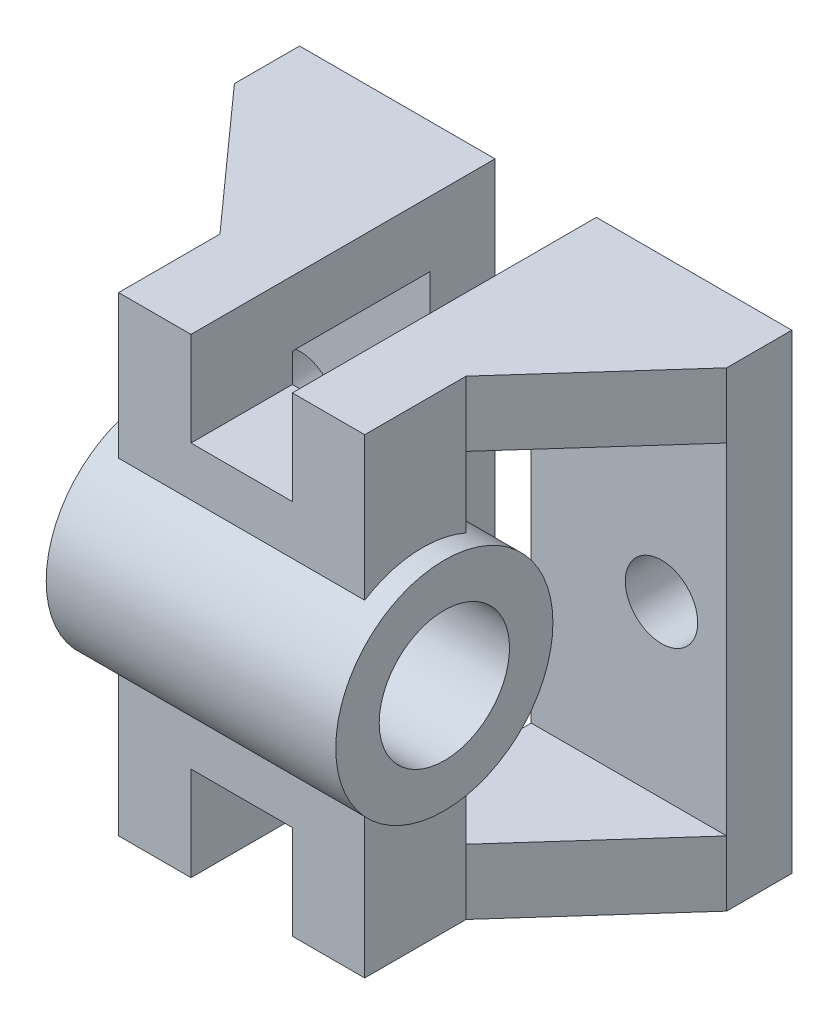
ISO-10303-21;
HEADER;
FILE_DESCRIPTION(('STEP AP214'),'2;1');
FILE_NAME('part.step','',(''),(''),'','','');
FILE_SCHEMA(('AUTOMOTIVE_DESIGN { 1 0 10303 214 1 1 1 1 }'));
ENDSEC;
DATA;
#1=APPLICATION_CONTEXT('core data for automotive mechanical design processes');
#2=APPLICATION_PROTOCOL_DEFINITION('international standard','automotive_design',2000,#1);
#3=PRODUCT_CONTEXT('',#1,'mechanical');
#4=PRODUCT('Part','Part','',(#3));
#5=PRODUCT_RELATED_PRODUCT_CATEGORY('part','',(#4));
#6=PRODUCT_DEFINITION_FORMATION('','',#4);
#7=PRODUCT_DEFINITION_CONTEXT('part definition',#1,'design');
#8=PRODUCT_DEFINITION('design','',#6,#7);
#9=PRODUCT_DEFINITION_SHAPE('','',#8);
#10=(LENGTH_UNIT() NAMED_UNIT(*) SI_UNIT(.MILLI.,.METRE.));
#11=(NAMED_UNIT(*) PLANE_ANGLE_UNIT() SI_UNIT($,.RADIAN.));
#12=(NAMED_UNIT(*) SI_UNIT($,.STERADIAN.) SOLID_ANGLE_UNIT());
#13=UNCERTAINTY_MEASURE_WITH_UNIT(LENGTH_MEASURE(1.E-05),#10,'distance_accuracy_value','');
#14=(GEOMETRIC_REPRESENTATION_CONTEXT(3) GLOBAL_UNCERTAINTY_ASSIGNED_CONTEXT((#13)) GLOBAL_UNIT_ASSIGNED_CONTEXT((#10,
#11,#12)) REPRESENTATION_CONTEXT('',''));
#15=CARTESIAN_POINT('',(0.,0.,0.));
#16=DIRECTION('',(0.,0.,1.));
#17=DIRECTION('',(1.,0.,0.));
#18=AXIS2_PLACEMENT_3D('',#15,#16,#17);
#19=CARTESIAN_POINT('',(17.,9.,42.));
#20=DIRECTION('',(-1.,0.,0.));
#21=DIRECTION('',(0.,0.,1.));
#22=AXIS2_PLACEMENT_3D('',#19,#20,#21);
#23=PLANE('',#22);
#24=DIRECTION('',(0.,-1.,0.));
#25=VECTOR('',#24,1.);
#26=CARTESIAN_POINT('',(17.,9.,42.));
#27=LINE('',#26,#25);
#28=CARTESIAN_POINT('',(17.,19.8114224595505,42.));
#29=VERTEX_POINT('',#28);
#30=CARTESIAN_POINT('',(17.,0.,42.));
#31=VERTEX_POINT('',#30);
#32=EDGE_CURVE('E248',#29,#31,#27,.T.);
#33=ORIENTED_EDGE('',*,*,#32,.F.);
#34=CARTESIAN_POINT('',(17.,32.5,34.));
#35=DIRECTION('',(-1.,0.,0.));
#36=DIRECTION('',(0.,0.,1.));
#37=AXIS2_PLACEMENT_3D('',#34,#35,#36);
#38=CIRCLE('',#37,15.);
#39=CARTESIAN_POINT('',(17.,18.7522729151325,28.));
#40=VERTEX_POINT('',#39);
#41=EDGE_CURVE('E64',#40,#29,#38,.T.);
#42=ORIENTED_EDGE('',*,*,#41,.F.);
#43=DIRECTION('',(0.,-1.,0.));
#44=VECTOR('',#43,1.);
#45=CARTESIAN_POINT('',(17.,65.,28.));
#46=LINE('',#45,#44);
#47=CARTESIAN_POINT('',(17.,9.,28.));
#48=VERTEX_POINT('',#47);
#49=EDGE_CURVE('E330',#40,#48,#46,.T.);
#50=ORIENTED_EDGE('',*,*,#49,.T.);
#51=DIRECTION('',(0.,-1.,0.));
#52=VECTOR('',#51,1.);
#53=CARTESIAN_POINT('',(17.,9.,28.));
#54=LINE('',#53,#52);
#55=CARTESIAN_POINT('',(17.,0.,28.));
#56=VERTEX_POINT('',#55);
#57=EDGE_CURVE('E243',#48,#56,#54,.T.);
#58=ORIENTED_EDGE('',*,*,#57,.T.);
#59=DIRECTION('',(0.,0.,-1.));
#60=VECTOR('',#59,1.);
#61=CARTESIAN_POINT('',(17.,0.,42.));
#62=LINE('',#61,#60);
#63=EDGE_CURVE('E387',#31,#56,#62,.T.);
#64=ORIENTED_EDGE('',*,*,#63,.F.);
#65=EDGE_LOOP('',(#33,#42,#50,#58,#64));
#66=FACE_BOUND('',#65,.T.);
#67=ADVANCED_FACE('F50',(#66),#23,.T.);
#68=CARTESIAN_POINT('',(17.,56.,28.));
#69=VERTEX_POINT('',#68);
#70=CARTESIAN_POINT('',(17.,46.2477270848675,28.));
#71=VERTEX_POINT('',#70);
#72=EDGE_CURVE('E261',#69,#71,#46,.T.);
#73=ORIENTED_EDGE('',*,*,#72,.T.);
#74=CARTESIAN_POINT('',(17.,45.1885775404495,42.));
#75=VERTEX_POINT('',#74);
#76=EDGE_CURVE('E252',#75,#71,#38,.T.);
#77=ORIENTED_EDGE('',*,*,#76,.F.);
#78=CARTESIAN_POINT('',(17.,65.,42.));
#79=VERTEX_POINT('',#78);
#80=EDGE_CURVE('E231',#79,#75,#27,.T.);
#81=ORIENTED_EDGE('',*,*,#80,.F.);
#82=DIRECTION('',(0.,0.,1.));
#83=VECTOR('',#82,1.);
#84=CARTESIAN_POINT('',(17.,65.,28.));
#85=LINE('',#84,#83);
#86=CARTESIAN_POINT('',(17.,65.,28.));
#87=VERTEX_POINT('',#86);
#88=EDGE_CURVE('E345',#87,#79,#85,.T.);
#89=ORIENTED_EDGE('',*,*,#88,.F.);
#90=DIRECTION('',(0.,1.,0.));
#91=VECTOR('',#90,1.);
#92=CARTESIAN_POINT('',(17.,56.,28.));
#93=LINE('',#92,#91);
#94=EDGE_CURVE('E363',#69,#87,#93,.T.);
#95=ORIENTED_EDGE('',*,*,#94,.F.);
#96=EDGE_LOOP('',(#73,#77,#81,#89,#95));
#97=FACE_BOUND('',#96,.T.);
#98=ADVANCED_FACE('F256',(#97),#23,.T.);
#99=CARTESIAN_POINT('',(51.,9.,42.));
#100=DIRECTION('',(1.,0.,0.));
#101=DIRECTION('',(0.,0.,-1.));
#102=AXIS2_PLACEMENT_3D('',#99,#100,#101);
#103=PLANE('',#102);
#104=CARTESIAN_POINT('',(51.,32.5,34.));
#105=DIRECTION('',(1.,0.,0.));
#106=DIRECTION('',(0.,0.,-1.));
#107=AXIS2_PLACEMENT_3D('',#104,#105,#106);
#108=CIRCLE('',#107,15.);
#109=CARTESIAN_POINT('',(51.,46.2477270848675,28.));
#110=VERTEX_POINT('',#109);
#111=CARTESIAN_POINT('',(51.,45.1885775404495,42.));
#112=VERTEX_POINT('',#111);
#113=EDGE_CURVE('E255',#110,#112,#108,.T.);
#114=ORIENTED_EDGE('',*,*,#113,.F.);
#115=DIRECTION('',(0.,-1.,0.));
#116=VECTOR('',#115,1.);
#117=CARTESIAN_POINT('',(51.,65.,28.));
#118=LINE('',#117,#116);
#119=CARTESIAN_POINT('',(51.,56.,28.));
#120=VERTEX_POINT('',#119);
#121=EDGE_CURVE('E327',#120,#110,#118,.T.);
#122=ORIENTED_EDGE('',*,*,#121,.F.);
#123=DIRECTION('',(0.,1.,0.));
#124=VECTOR('',#123,1.);
#125=CARTESIAN_POINT('',(51.,56.,28.));
#126=LINE('',#125,#124);
#127=CARTESIAN_POINT('',(51.,65.,28.));
#128=VERTEX_POINT('',#127);
#129=EDGE_CURVE('E349',#120,#128,#126,.T.);
#130=ORIENTED_EDGE('',*,*,#129,.T.);
#131=DIRECTION('',(0.,0.,-1.));
#132=VECTOR('',#131,1.);
#133=CARTESIAN_POINT('',(51.,65.,42.));
#134=LINE('',#133,#132);
#135=CARTESIAN_POINT('',(51.,65.,42.));
#136=VERTEX_POINT('',#135);
#137=EDGE_CURVE('E352',#136,#128,#134,.T.);
#138=ORIENTED_EDGE('',*,*,#137,.F.);
#139=DIRECTION('',(0.,-1.,0.));
#140=VECTOR('',#139,1.);
#141=CARTESIAN_POINT('',(51.,9.,42.));
#142=LINE('',#141,#140);
#143=EDGE_CURVE('E399',#136,#112,#142,.T.);
#144=ORIENTED_EDGE('',*,*,#143,.T.);
#145=EDGE_LOOP('',(#114,#122,#130,#138,#144));
#146=FACE_BOUND('',#145,.T.);
#147=ADVANCED_FACE('F454',(#146),#103,.T.);
#148=CARTESIAN_POINT('',(34.,9.,42.));
#149=DIRECTION('',(0.,0.,1.));
#150=DIRECTION('',(1.,0.,0.));
#151=AXIS2_PLACEMENT_3D('',#148,#149,#150);
#152=PLANE('',#151);
#153=DIRECTION('',(-1.,0.,0.));
#154=VECTOR('',#153,1.);
#155=CARTESIAN_POINT('',(54.,45.1885775404495,42.));
#156=LINE('',#155,#154);
#157=EDGE_CURVE('E240',#112,#75,#156,.T.);
#158=ORIENTED_EDGE('',*,*,#157,.F.);
#159=ORIENTED_EDGE('',*,*,#143,.F.);
#160=DIRECTION('',(1.,0.,0.));
#161=VECTOR('',#160,1.);
#162=CARTESIAN_POINT('',(34.,65.,42.));
#163=LINE('',#162,#161);
#164=CARTESIAN_POINT('',(41.,65.,42.));
#165=VERTEX_POINT('',#164);
#166=EDGE_CURVE('E339',#165,#136,#163,.T.);
#167=ORIENTED_EDGE('',*,*,#166,.F.);
#168=DIRECTION('',(0.,1.,0.));
#169=VECTOR('',#168,1.);
#170=CARTESIAN_POINT('',(41.,52.,42.));
#171=LINE('',#170,#169);
#172=CARTESIAN_POINT('',(41.,52.,42.));
#173=VERTEX_POINT('',#172);
#174=EDGE_CURVE('E285',#173,#165,#171,.T.);
#175=ORIENTED_EDGE('',*,*,#174,.F.);
#176=DIRECTION('',(1.,0.,0.));
#177=VECTOR('',#176,1.);
#178=CARTESIAN_POINT('',(27.,52.,42.));
#179=LINE('',#178,#177);
#180=CARTESIAN_POINT('',(27.,52.,42.));
#181=VERTEX_POINT('',#180);
#182=EDGE_CURVE('E277',#181,#173,#179,.T.);
#183=ORIENTED_EDGE('',*,*,#182,.F.);
#184=DIRECTION('',(0.,1.,0.));
#185=VECTOR('',#184,1.);
#186=CARTESIAN_POINT('',(27.,52.,42.));
#187=LINE('',#186,#185);
#188=CARTESIAN_POINT('',(27.,65.,42.));
#189=VERTEX_POINT('',#188);
#190=EDGE_CURVE('E67',#181,#189,#187,.T.);
#191=ORIENTED_EDGE('',*,*,#190,.T.);
#192=EDGE_CURVE('E238',#79,#189,#163,.T.);
#193=ORIENTED_EDGE('',*,*,#192,.F.);
#194=ORIENTED_EDGE('',*,*,#80,.T.);
#195=EDGE_LOOP('',(#158,#159,#167,#175,#183,#191,#193,#194));
#196=FACE_BOUND('',#195,.T.);
#197=ADVANCED_FACE('F234',(#196),#152,.T.);
#198=CARTESIAN_POINT('',(17.,65.,28.));
#199=DIRECTION('',(0.,0.,-1.));
#200=DIRECTION('',(-1.,0.,0.));
#201=AXIS2_PLACEMENT_3D('',#198,#199,#200);
#202=PLANE('',#201);
#203=DIRECTION('',(-1.,0.,0.));
#204=VECTOR('',#203,1.);
#205=CARTESIAN_POINT('',(54.,18.7522729151325,28.));
#206=LINE('',#205,#204);
#207=CARTESIAN_POINT('',(51.,18.7522729151325,28.));
#208=VERTEX_POINT('',#207);
#209=EDGE_CURVE('E11',#208,#40,#206,.T.);
#210=ORIENTED_EDGE('',*,*,#209,.F.);
#211=CARTESIAN_POINT('',(51.,9.,28.));
#212=VERTEX_POINT('',#211);
#213=EDGE_CURVE('E335',#208,#212,#118,.T.);
#214=ORIENTED_EDGE('',*,*,#213,.T.);
#215=DIRECTION('',(1.,0.,0.));
#216=VECTOR('',#215,1.);
#217=CARTESIAN_POINT('',(0.,9.,28.));
#218=LINE('',#217,#216);
#219=CARTESIAN_POINT('',(41.,9.,28.));
#220=VERTEX_POINT('',#219);
#221=EDGE_CURVE('E332',#220,#212,#218,.T.);
#222=ORIENTED_EDGE('',*,*,#221,.F.);
#223=DIRECTION('',(0.,-1.,0.));
#224=VECTOR('',#223,1.);
#225=CARTESIAN_POINT('',(41.,65.,28.));
#226=LINE('',#225,#224);
#227=CARTESIAN_POINT('',(41.,13.,28.));
#228=VERTEX_POINT('',#227);
#229=EDGE_CURVE('E444',#228,#220,#226,.T.);
#230=ORIENTED_EDGE('',*,*,#229,.F.);
#231=DIRECTION('',(1.,0.,0.));
#232=VECTOR('',#231,1.);
#233=CARTESIAN_POINT('',(17.,13.,28.));
#234=LINE('',#233,#232);
#235=CARTESIAN_POINT('',(27.,13.,28.));
#236=VERTEX_POINT('',#235);
#237=EDGE_CURVE('E437',#236,#228,#234,.T.);
#238=ORIENTED_EDGE('',*,*,#237,.F.);
#239=DIRECTION('',(0.,1.,0.));
#240=VECTOR('',#239,1.);
#241=CARTESIAN_POINT('',(27.,65.,28.));
#242=LINE('',#241,#240);
#243=CARTESIAN_POINT('',(27.,9.,28.));
#244=VERTEX_POINT('',#243);
#245=EDGE_CURVE('E439',#244,#236,#242,.T.);
#246=ORIENTED_EDGE('',*,*,#245,.F.);
#247=EDGE_CURVE('E331',#48,#244,#218,.T.);
#248=ORIENTED_EDGE('',*,*,#247,.F.);
#249=ORIENTED_EDGE('',*,*,#49,.F.);
#250=EDGE_LOOP('',(#210,#214,#222,#230,#238,#246,#248,#249));
#251=FACE_BOUND('',#250,.T.);
#252=ADVANCED_FACE('F523',(#251),#202,.T.);
#253=CARTESIAN_POINT('',(0.,0.,9.));
#254=DIRECTION('',(0.,0.,1.));
#255=DIRECTION('',(1.,0.,0.));
#256=AXIS2_PLACEMENT_3D('',#253,#254,#255);
#257=PLANE('',#256);
#258=CARTESIAN_POINT('',(8.99999999999999,32.5,9.));
#259=DIRECTION('',(0.,0.,-1.));
#260=DIRECTION('',(-1.,0.,0.));
#261=AXIS2_PLACEMENT_3D('',#258,#259,#260);
#262=CIRCLE('',#261,5.);
#263=CARTESIAN_POINT('',(3.99999999999999,32.5,9.));
#264=VERTEX_POINT('',#263);
#265=EDGE_CURVE('E1003',#264,#264,#262,.T.);
#266=ORIENTED_EDGE('',*,*,#265,.T.);
#267=EDGE_LOOP('',(#266));
#268=FACE_BOUND('',#267,.T.);
#269=DIRECTION('',(0.,-1.,0.));
#270=VECTOR('',#269,1.);
#271=CARTESIAN_POINT('',(27.,0.,9.));
#272=LINE('',#271,#270);
#273=CARTESIAN_POINT('',(27.,56.,9.));
#274=VERTEX_POINT('',#273);
#275=CARTESIAN_POINT('',(27.,9.,9.));
#276=VERTEX_POINT('',#275);
#277=EDGE_CURVE('E319',#274,#276,#272,.T.);
#278=ORIENTED_EDGE('',*,*,#277,.F.);
#279=DIRECTION('',(-1.,0.,0.));
#280=VECTOR('',#279,1.);
#281=CARTESIAN_POINT('',(68.,56.,9.));
#282=LINE('',#281,#280);
#283=CARTESIAN_POINT('',(0.,56.,9.));
#284=VERTEX_POINT('',#283);
#285=EDGE_CURVE('E343',#274,#284,#282,.T.);
#286=ORIENTED_EDGE('',*,*,#285,.T.);
#287=DIRECTION('',(0.,-1.,0.));
#288=VECTOR('',#287,1.);
#289=CARTESIAN_POINT('',(0.,65.,9.));
#290=LINE('',#289,#288);
#291=CARTESIAN_POINT('',(0.,9.,9.));
#292=VERTEX_POINT('',#291);
#293=EDGE_CURVE('E407',#284,#292,#290,.T.);
#294=ORIENTED_EDGE('',*,*,#293,.T.);
#295=DIRECTION('',(1.,0.,0.));
#296=VECTOR('',#295,1.);
#297=CARTESIAN_POINT('',(0.,9.,9.));
#298=LINE('',#297,#296);
#299=EDGE_CURVE('E373',#292,#276,#298,.T.);
#300=ORIENTED_EDGE('',*,*,#299,.T.);
#301=EDGE_LOOP('',(#278,#286,#294,#300));
#302=FACE_BOUND('',#301,.T.);
#303=ADVANCED_FACE('F492',(#268,#302),#257,.T.);
#304=CARTESIAN_POINT('',(0.,0.,0.));
#305=DIRECTION('',(0.,0.,1.));
#306=DIRECTION('',(1.,0.,0.));
#307=AXIS2_PLACEMENT_3D('',#304,#305,#306);
#308=PLANE('',#307);
#309=CARTESIAN_POINT('',(8.99999999999999,32.5,0.));
#310=DIRECTION('',(0.,0.,-1.));
#311=DIRECTION('',(-1.,0.,0.));
#312=AXIS2_PLACEMENT_3D('',#309,#310,#311);
#313=CIRCLE('',#312,5.);
#314=CARTESIAN_POINT('',(3.99999999999999,32.5,0.));
#315=VERTEX_POINT('',#314);
#316=EDGE_CURVE('E1000',#315,#315,#313,.T.);
#317=ORIENTED_EDGE('',*,*,#316,.F.);
#318=EDGE_LOOP('',(#317));
#319=FACE_BOUND('',#318,.T.);
#320=DIRECTION('',(-1.,0.,0.));
#321=VECTOR('',#320,1.);
#322=CARTESIAN_POINT('',(68.,65.,0.));
#323=LINE('',#322,#321);
#324=CARTESIAN_POINT('',(27.,65.,0.));
#325=VERTEX_POINT('',#324);
#326=CARTESIAN_POINT('',(0.,65.,0.));
#327=VERTEX_POINT('',#326);
#328=EDGE_CURVE('E420',#325,#327,#323,.T.);
#329=ORIENTED_EDGE('',*,*,#328,.F.);
#330=DIRECTION('',(0.,-1.,0.));
#331=VECTOR('',#330,1.);
#332=CARTESIAN_POINT('',(27.,13.,0.));
#333=LINE('',#332,#331);
#334=CARTESIAN_POINT('',(27.,0.,0.));
#335=VERTEX_POINT('',#334);
#336=EDGE_CURVE('E314',#325,#335,#333,.T.);
#337=ORIENTED_EDGE('',*,*,#336,.T.);
#338=DIRECTION('',(1.,0.,0.));
#339=VECTOR('',#338,1.);
#340=CARTESIAN_POINT('',(0.,0.,0.));
#341=LINE('',#340,#339);
#342=CARTESIAN_POINT('',(0.,0.,0.));
#343=VERTEX_POINT('',#342);
#344=EDGE_CURVE('E412',#343,#335,#341,.T.);
#345=ORIENTED_EDGE('',*,*,#344,.F.);
#346=DIRECTION('',(0.,-1.,0.));
#347=VECTOR('',#346,1.);
#348=CARTESIAN_POINT('',(0.,65.,0.));
#349=LINE('',#348,#347);
#350=EDGE_CURVE('E398',#327,#343,#349,.T.);
#351=ORIENTED_EDGE('',*,*,#350,.F.);
#352=EDGE_LOOP('',(#329,#337,#345,#351));
#353=FACE_BOUND('',#352,.T.);
#354=ADVANCED_FACE('F506',(#319,#353),#308,.F.);
#355=CARTESIAN_POINT('',(68.,65.,9.));
#356=DIRECTION('',(0.,-1.,0.));
#357=DIRECTION('',(0.,0.,-1.));
#358=AXIS2_PLACEMENT_3D('',#355,#356,#357);
#359=PLANE('',#358);
#360=ORIENTED_EDGE('',*,*,#192,.T.);
#361=DIRECTION('',(0.,0.,1.));
#362=VECTOR('',#361,1.);
#363=CARTESIAN_POINT('',(27.,65.,0.));
#364=LINE('',#363,#362);
#365=EDGE_CURVE('E276',#325,#189,#364,.T.);
#366=ORIENTED_EDGE('',*,*,#365,.F.);
#367=ORIENTED_EDGE('',*,*,#328,.T.);
#368=DIRECTION('',(0.,0.,-1.));
#369=VECTOR('',#368,1.);
#370=CARTESIAN_POINT('',(0.,65.,9.));
#371=LINE('',#370,#369);
#372=CARTESIAN_POINT('',(0.,65.,9.));
#373=VERTEX_POINT('',#372);
#374=EDGE_CURVE('E408',#373,#327,#371,.T.);
#375=ORIENTED_EDGE('',*,*,#374,.F.);
#376=DIRECTION('',(0.666794859469826,0.,0.745241313525099));
#377=VECTOR('',#376,1.);
#378=CARTESIAN_POINT('',(0.,65.,9.));
#379=LINE('',#378,#377);
#380=EDGE_CURVE('E360',#373,#87,#379,.T.);
#381=ORIENTED_EDGE('',*,*,#380,.T.);
#382=ORIENTED_EDGE('',*,*,#88,.T.);
#383=EDGE_LOOP('',(#360,#366,#367,#375,#381,#382));
#384=FACE_BOUND('',#383,.T.);
#385=ADVANCED_FACE('F505',(#384),#359,.F.);
#386=CARTESIAN_POINT('',(0.,56.,0.));
#387=DIRECTION('',(0.,1.,0.));
#388=DIRECTION('',(0.,0.,1.));
#389=AXIS2_PLACEMENT_3D('',#386,#387,#388);
#390=PLANE('',#389);
#391=ORIENTED_EDGE('',*,*,#285,.F.);
#392=DIRECTION('',(0.,0.,1.));
#393=VECTOR('',#392,1.);
#394=CARTESIAN_POINT('',(27.,56.,0.));
#395=LINE('',#394,#393);
#396=CARTESIAN_POINT('',(27.,56.,28.));
#397=VERTEX_POINT('',#396);
#398=EDGE_CURVE('E295',#274,#397,#395,.T.);
#399=ORIENTED_EDGE('',*,*,#398,.T.);
#400=DIRECTION('',(-1.,0.,0.));
#401=VECTOR('',#400,1.);
#402=CARTESIAN_POINT('',(0.,56.,28.));
#403=LINE('',#402,#401);
#404=EDGE_CURVE('E432',#397,#69,#403,.T.);
#405=ORIENTED_EDGE('',*,*,#404,.T.);
#406=DIRECTION('',(0.666794859469826,0.,0.745241313525099));
#407=VECTOR('',#406,1.);
#408=CARTESIAN_POINT('',(0.,56.,9.));
#409=LINE('',#408,#407);
#410=EDGE_CURVE('E347',#284,#69,#409,.T.);
#411=ORIENTED_EDGE('',*,*,#410,.F.);
#412=EDGE_LOOP('',(#391,#399,#405,#411));
#413=FACE_BOUND('',#412,.T.);
#414=ADVANCED_FACE('F484',(#413),#390,.F.);
#415=CARTESIAN_POINT('',(0.,0.,9.));
#416=DIRECTION('',(0.,1.,0.));
#417=DIRECTION('',(0.,0.,1.));
#418=AXIS2_PLACEMENT_3D('',#415,#416,#417);
#419=PLANE('',#418);
#420=DIRECTION('',(-1.,0.,0.));
#421=VECTOR('',#420,1.);
#422=CARTESIAN_POINT('',(34.,0.,42.));
#423=LINE('',#422,#421);
#424=CARTESIAN_POINT('',(51.,0.,42.));
#425=VERTEX_POINT('',#424);
#426=CARTESIAN_POINT('',(41.,0.,42.));
#427=VERTEX_POINT('',#426);
#428=EDGE_CURVE('E382',#425,#427,#423,.T.);
#429=ORIENTED_EDGE('',*,*,#428,.T.);
#430=DIRECTION('',(0.,0.,1.));
#431=VECTOR('',#430,1.);
#432=CARTESIAN_POINT('',(41.,0.,42.));
#433=LINE('',#432,#431);
#434=CARTESIAN_POINT('',(41.,0.,0.));
#435=VERTEX_POINT('',#434);
#436=EDGE_CURVE('E298',#435,#427,#433,.T.);
#437=ORIENTED_EDGE('',*,*,#436,.F.);
#438=CARTESIAN_POINT('',(68.,0.,0.));
#439=VERTEX_POINT('',#438);
#440=EDGE_CURVE('E411',#435,#439,#341,.T.);
#441=ORIENTED_EDGE('',*,*,#440,.T.);
#442=DIRECTION('',(0.,0.,-1.));
#443=VECTOR('',#442,1.);
#444=CARTESIAN_POINT('',(68.,0.,9.));
#445=LINE('',#444,#443);
#446=CARTESIAN_POINT('',(68.,0.,9.));
#447=VERTEX_POINT('',#446);
#448=EDGE_CURVE('E428',#447,#439,#445,.T.);
#449=ORIENTED_EDGE('',*,*,#448,.F.);
#450=DIRECTION('',(-0.666794859469826,0.,0.745241313525099));
#451=VECTOR('',#450,1.);
#452=CARTESIAN_POINT('',(51.,0.,28.));
#453=LINE('',#452,#451);
#454=CARTESIAN_POINT('',(51.,0.,28.));
#455=VERTEX_POINT('',#454);
#456=EDGE_CURVE('E375',#447,#455,#453,.T.);
#457=ORIENTED_EDGE('',*,*,#456,.T.);
#458=DIRECTION('',(0.,0.,1.));
#459=VECTOR('',#458,1.);
#460=CARTESIAN_POINT('',(51.,0.,42.));
#461=LINE('',#460,#459);
#462=EDGE_CURVE('E361',#455,#425,#461,.T.);
#463=ORIENTED_EDGE('',*,*,#462,.T.);
#464=EDGE_LOOP('',(#429,#437,#441,#449,#457,#463));
#465=FACE_BOUND('',#464,.T.);
#466=ADVANCED_FACE('F553',(#465),#419,.F.);
#467=CARTESIAN_POINT('',(0.,9.,0.));
#468=DIRECTION('',(0.,-1.,0.));
#469=DIRECTION('',(0.,0.,-1.));
#470=AXIS2_PLACEMENT_3D('',#467,#468,#469);
#471=PLANE('',#470);
#472=CARTESIAN_POINT('',(41.,9.,9.));
#473=VERTEX_POINT('',#472);
#474=CARTESIAN_POINT('',(68.,9.,9.));
#475=VERTEX_POINT('',#474);
#476=EDGE_CURVE('E371',#473,#475,#298,.T.);
#477=ORIENTED_EDGE('',*,*,#476,.F.);
#478=DIRECTION('',(0.,0.,1.));
#479=VECTOR('',#478,1.);
#480=CARTESIAN_POINT('',(41.,9.,0.));
#481=LINE('',#480,#479);
#482=EDGE_CURVE('E325',#473,#220,#481,.T.);
#483=ORIENTED_EDGE('',*,*,#482,.T.);
#484=ORIENTED_EDGE('',*,*,#221,.T.);
#485=DIRECTION('',(-0.666794859469826,0.,0.745241313525099));
#486=VECTOR('',#485,1.);
#487=CARTESIAN_POINT('',(51.,9.,28.));
#488=LINE('',#487,#486);
#489=EDGE_CURVE('E376',#475,#212,#488,.T.);
#490=ORIENTED_EDGE('',*,*,#489,.F.);
#491=EDGE_LOOP('',(#477,#483,#484,#490));
#492=FACE_BOUND('',#491,.T.);
#493=ADVANCED_FACE('F549',(#492),#471,.F.);
#494=CARTESIAN_POINT('',(59.,32.5,9.));
#495=DIRECTION('',(0.,0.,-1.));
#496=DIRECTION('',(-1.,0.,0.));
#497=AXIS2_PLACEMENT_3D('',#494,#495,#496);
#498=CIRCLE('',#497,5.00000000000001);
#499=CARTESIAN_POINT('',(54.,32.5,9.));
#500=VERTEX_POINT('',#499);
#501=EDGE_CURVE('E993',#500,#500,#498,.T.);
#502=ORIENTED_EDGE('',*,*,#501,.T.);
#503=EDGE_LOOP('',(#502));
#504=FACE_BOUND('',#503,.T.);
#505=CARTESIAN_POINT('',(68.,56.,9.));
#506=VERTEX_POINT('',#505);
#507=CARTESIAN_POINT('',(41.,56.,9.));
#508=VERTEX_POINT('',#507);
#509=EDGE_CURVE('E341',#506,#508,#282,.T.);
#510=ORIENTED_EDGE('',*,*,#509,.T.);
#511=DIRECTION('',(0.,1.,0.));
#512=VECTOR('',#511,1.);
#513=CARTESIAN_POINT('',(41.,0.,9.));
#514=LINE('',#513,#512);
#515=EDGE_CURVE('E324',#473,#508,#514,.T.);
#516=ORIENTED_EDGE('',*,*,#515,.F.);
#517=ORIENTED_EDGE('',*,*,#476,.T.);
#518=DIRECTION('',(0.,1.,0.));
#519=VECTOR('',#518,1.);
#520=CARTESIAN_POINT('',(68.,0.,9.));
#521=LINE('',#520,#519);
#522=EDGE_CURVE('E403',#475,#506,#521,.T.);
#523=ORIENTED_EDGE('',*,*,#522,.T.);
#524=EDGE_LOOP('',(#510,#516,#517,#523));
#525=FACE_BOUND('',#524,.T.);
#526=ADVANCED_FACE('F561',(#504,#525),#257,.T.);
#527=CARTESIAN_POINT('',(0.,65.,9.));
#528=DIRECTION('',(1.,0.,0.));
#529=DIRECTION('',(0.,0.,-1.));
#530=AXIS2_PLACEMENT_3D('',#527,#528,#529);
#531=PLANE('',#530);
#532=ORIENTED_EDGE('',*,*,#350,.T.);
#533=DIRECTION('',(0.,0.,-1.));
#534=VECTOR('',#533,1.);
#535=CARTESIAN_POINT('',(0.,0.,9.));
#536=LINE('',#535,#534);
#537=CARTESIAN_POINT('',(0.,0.,9.));
#538=VERTEX_POINT('',#537);
#539=EDGE_CURVE('E431',#538,#343,#536,.T.);
#540=ORIENTED_EDGE('',*,*,#539,.F.);
#541=DIRECTION('',(0.,-1.,0.));
#542=VECTOR('',#541,1.);
#543=CARTESIAN_POINT('',(0.,9.,9.));
#544=LINE('',#543,#542);
#545=EDGE_CURVE('E400',#292,#538,#544,.T.);
#546=ORIENTED_EDGE('',*,*,#545,.F.);
#547=ORIENTED_EDGE('',*,*,#293,.F.);
#548=EDGE_CURVE('E405',#373,#284,#290,.T.);
#549=ORIENTED_EDGE('',*,*,#548,.F.);
#550=ORIENTED_EDGE('',*,*,#374,.T.);
#551=EDGE_LOOP('',(#532,#540,#546,#547,#549,#550));
#552=FACE_BOUND('',#551,.T.);
#553=ADVANCED_FACE('F47',(#552),#531,.F.);
#554=ORIENTED_EDGE('',*,*,#344,.T.);
#555=DIRECTION('',(0.,0.,-1.));
#556=VECTOR('',#555,1.);
#557=CARTESIAN_POINT('',(27.,0.,0.));
#558=LINE('',#557,#556);
#559=CARTESIAN_POINT('',(27.,0.,42.));
#560=VERTEX_POINT('',#559);
#561=EDGE_CURVE('E293',#560,#335,#558,.T.);
#562=ORIENTED_EDGE('',*,*,#561,.F.);
#563=EDGE_CURVE('E385',#560,#31,#423,.T.);
#564=ORIENTED_EDGE('',*,*,#563,.T.);
#565=ORIENTED_EDGE('',*,*,#63,.T.);
#566=DIRECTION('',(-0.666794859469826,0.,-0.745241313525099));
#567=VECTOR('',#566,1.);
#568=CARTESIAN_POINT('',(17.,0.,28.));
#569=LINE('',#568,#567);
#570=EDGE_CURVE('E386',#56,#538,#569,.T.);
#571=ORIENTED_EDGE('',*,*,#570,.T.);
#572=ORIENTED_EDGE('',*,*,#539,.T.);
#573=EDGE_LOOP('',(#554,#562,#564,#565,#571,#572));
#574=FACE_BOUND('',#573,.T.);
#575=ADVANCED_FACE('F512',(#574),#419,.F.);
#576=CARTESIAN_POINT('',(68.,0.,9.));
#577=DIRECTION('',(-1.,0.,0.));
#578=DIRECTION('',(0.,0.,1.));
#579=AXIS2_PLACEMENT_3D('',#576,#577,#578);
#580=PLANE('',#579);
#581=DIRECTION('',(0.,1.,0.));
#582=VECTOR('',#581,1.);
#583=CARTESIAN_POINT('',(68.,0.,0.));
#584=LINE('',#583,#582);
#585=CARTESIAN_POINT('',(68.,65.,0.));
#586=VERTEX_POINT('',#585);
#587=EDGE_CURVE('E417',#439,#586,#584,.T.);
#588=ORIENTED_EDGE('',*,*,#587,.T.);
#589=DIRECTION('',(0.,0.,-1.));
#590=VECTOR('',#589,1.);
#591=CARTESIAN_POINT('',(68.,65.,9.));
#592=LINE('',#591,#590);
#593=CARTESIAN_POINT('',(68.,65.,9.));
#594=VERTEX_POINT('',#593);
#595=EDGE_CURVE('E422',#594,#586,#592,.T.);
#596=ORIENTED_EDGE('',*,*,#595,.F.);
#597=DIRECTION('',(0.,1.,0.));
#598=VECTOR('',#597,1.);
#599=CARTESIAN_POINT('',(68.,56.,9.));
#600=LINE('',#599,#598);
#601=EDGE_CURVE('E365',#506,#594,#600,.T.);
#602=ORIENTED_EDGE('',*,*,#601,.F.);
#603=ORIENTED_EDGE('',*,*,#522,.F.);
#604=EDGE_CURVE('E409',#447,#475,#521,.T.);
#605=ORIENTED_EDGE('',*,*,#604,.F.);
#606=ORIENTED_EDGE('',*,*,#448,.T.);
#607=EDGE_LOOP('',(#588,#596,#602,#603,#605,#606));
#608=FACE_BOUND('',#607,.T.);
#609=ADVANCED_FACE('F558',(#608),#580,.F.);
#610=CARTESIAN_POINT('',(41.,65.,0.));
#611=VERTEX_POINT('',#610);
#612=EDGE_CURVE('E419',#586,#611,#323,.T.);
#613=ORIENTED_EDGE('',*,*,#612,.T.);
#614=DIRECTION('',(0.,0.,-1.));
#615=VECTOR('',#614,1.);
#616=CARTESIAN_POINT('',(41.,65.,42.));
#617=LINE('',#616,#615);
#618=EDGE_CURVE('E274',#165,#611,#617,.T.);
#619=ORIENTED_EDGE('',*,*,#618,.F.);
#620=ORIENTED_EDGE('',*,*,#166,.T.);
#621=ORIENTED_EDGE('',*,*,#137,.T.);
#622=DIRECTION('',(0.666794859469826,0.,-0.745241313525099));
#623=VECTOR('',#622,1.);
#624=CARTESIAN_POINT('',(51.,65.,28.));
#625=LINE('',#624,#623);
#626=EDGE_CURVE('E351',#128,#594,#625,.T.);
#627=ORIENTED_EDGE('',*,*,#626,.T.);
#628=ORIENTED_EDGE('',*,*,#595,.T.);
#629=EDGE_LOOP('',(#613,#619,#620,#621,#627,#628));
#630=FACE_BOUND('',#629,.T.);
#631=ADVANCED_FACE('F466',(#630),#359,.F.);
#632=CARTESIAN_POINT('',(59.,32.5,0.));
#633=DIRECTION('',(0.,0.,-1.));
#634=DIRECTION('',(-1.,0.,0.));
#635=AXIS2_PLACEMENT_3D('',#632,#633,#634);
#636=CIRCLE('',#635,5.00000000000001);
#637=CARTESIAN_POINT('',(54.,32.5,0.));
#638=VERTEX_POINT('',#637);
#639=EDGE_CURVE('E1002',#638,#638,#636,.T.);
#640=ORIENTED_EDGE('',*,*,#639,.F.);
#641=EDGE_LOOP('',(#640));
#642=FACE_BOUND('',#641,.T.);
#643=DIRECTION('',(0.,-1.,0.));
#644=VECTOR('',#643,1.);
#645=CARTESIAN_POINT('',(41.,13.,0.));
#646=LINE('',#645,#644);
#647=EDGE_CURVE('E315',#611,#435,#646,.T.);
#648=ORIENTED_EDGE('',*,*,#647,.F.);
#649=ORIENTED_EDGE('',*,*,#612,.F.);
#650=ORIENTED_EDGE('',*,*,#587,.F.);
#651=ORIENTED_EDGE('',*,*,#440,.F.);
#652=EDGE_LOOP('',(#648,#649,#650,#651));
#653=FACE_BOUND('',#652,.T.);
#654=ADVANCED_FACE('F589',(#642,#653),#308,.F.);
#655=CARTESIAN_POINT('',(51.,19.8114224595505,42.));
#656=VERTEX_POINT('',#655);
#657=EDGE_CURVE('E254',#656,#208,#108,.T.);
#658=ORIENTED_EDGE('',*,*,#657,.F.);
#659=EDGE_CURVE('E377',#656,#425,#142,.T.);
#660=ORIENTED_EDGE('',*,*,#659,.T.);
#661=ORIENTED_EDGE('',*,*,#462,.F.);
#662=DIRECTION('',(0.,-1.,0.));
#663=VECTOR('',#662,1.);
#664=CARTESIAN_POINT('',(51.,9.,28.));
#665=LINE('',#664,#663);
#666=EDGE_CURVE('E391',#212,#455,#665,.T.);
#667=ORIENTED_EDGE('',*,*,#666,.F.);
#668=ORIENTED_EDGE('',*,*,#213,.F.);
#669=EDGE_LOOP('',(#658,#660,#661,#667,#668));
#670=FACE_BOUND('',#669,.T.);
#671=ADVANCED_FACE('F541',(#670),#103,.T.);
#672=CARTESIAN_POINT('',(51.,9.,28.));
#673=DIRECTION('',(0.745241313525099,0.,0.666794859469826));
#674=DIRECTION('',(0.666794859469826,0.,-0.745241313525099));
#675=AXIS2_PLACEMENT_3D('',#672,#673,#674);
#676=PLANE('',#675);
#677=ORIENTED_EDGE('',*,*,#456,.F.);
#678=ORIENTED_EDGE('',*,*,#604,.T.);
#679=ORIENTED_EDGE('',*,*,#489,.T.);
#680=ORIENTED_EDGE('',*,*,#666,.T.);
#681=EDGE_LOOP('',(#677,#678,#679,#680));
#682=FACE_BOUND('',#681,.T.);
#683=ADVANCED_FACE('F544',(#682),#676,.T.);
#684=CARTESIAN_POINT('',(17.,9.,28.));
#685=DIRECTION('',(-0.745241313525099,0.,0.666794859469826));
#686=DIRECTION('',(0.666794859469826,0.,0.745241313525099));
#687=AXIS2_PLACEMENT_3D('',#684,#685,#686);
#688=PLANE('',#687);
#689=ORIENTED_EDGE('',*,*,#570,.F.);
#690=ORIENTED_EDGE('',*,*,#57,.F.);
#691=DIRECTION('',(-0.666794859469826,0.,-0.745241313525099));
#692=VECTOR('',#691,1.);
#693=CARTESIAN_POINT('',(17.,9.,28.));
#694=LINE('',#693,#692);
#695=EDGE_CURVE('E366',#48,#292,#694,.T.);
#696=ORIENTED_EDGE('',*,*,#695,.T.);
#697=ORIENTED_EDGE('',*,*,#545,.T.);
#698=EDGE_LOOP('',(#689,#690,#696,#697));
#699=FACE_BOUND('',#698,.T.);
#700=ADVANCED_FACE('F519',(#699),#688,.T.);
#701=DIRECTION('',(-1.,0.,0.));
#702=VECTOR('',#701,1.);
#703=CARTESIAN_POINT('',(54.,19.8114224595505,42.));
#704=LINE('',#703,#702);
#705=EDGE_CURVE('E272',#29,#656,#704,.F.);
#706=ORIENTED_EDGE('',*,*,#705,.F.);
#707=ORIENTED_EDGE('',*,*,#32,.T.);
#708=ORIENTED_EDGE('',*,*,#563,.F.);
#709=DIRECTION('',(0.,-1.,0.));
#710=VECTOR('',#709,1.);
#711=CARTESIAN_POINT('',(27.,13.,42.));
#712=LINE('',#711,#710);
#713=CARTESIAN_POINT('',(27.,13.,42.));
#714=VERTEX_POINT('',#713);
#715=EDGE_CURVE('E304',#714,#560,#712,.T.);
#716=ORIENTED_EDGE('',*,*,#715,.F.);
#717=DIRECTION('',(-1.,0.,0.));
#718=VECTOR('',#717,1.);
#719=CARTESIAN_POINT('',(27.,13.,42.));
#720=LINE('',#719,#718);
#721=CARTESIAN_POINT('',(41.,13.,42.));
#722=VERTEX_POINT('',#721);
#723=EDGE_CURVE('E297',#722,#714,#720,.T.);
#724=ORIENTED_EDGE('',*,*,#723,.F.);
#725=DIRECTION('',(0.,-1.,0.));
#726=VECTOR('',#725,1.);
#727=CARTESIAN_POINT('',(41.,13.,42.));
#728=LINE('',#727,#726);
#729=EDGE_CURVE('E306',#722,#427,#728,.T.);
#730=ORIENTED_EDGE('',*,*,#729,.T.);
#731=ORIENTED_EDGE('',*,*,#428,.F.);
#732=ORIENTED_EDGE('',*,*,#659,.F.);
#733=EDGE_LOOP('',(#706,#707,#708,#716,#724,#730,#731,#732));
#734=FACE_BOUND('',#733,.T.);
#735=ADVANCED_FACE('F533',(#734),#152,.T.);
#736=ORIENTED_EDGE('',*,*,#247,.T.);
#737=DIRECTION('',(0.,0.,-1.));
#738=VECTOR('',#737,1.);
#739=CARTESIAN_POINT('',(27.,9.,0.));
#740=LINE('',#739,#738);
#741=EDGE_CURVE('E313',#244,#276,#740,.T.);
#742=ORIENTED_EDGE('',*,*,#741,.T.);
#743=ORIENTED_EDGE('',*,*,#299,.F.);
#744=ORIENTED_EDGE('',*,*,#695,.F.);
#745=EDGE_LOOP('',(#736,#742,#743,#744));
#746=FACE_BOUND('',#745,.T.);
#747=ADVANCED_FACE('F489',(#746),#471,.F.);
#748=CARTESIAN_POINT('',(0.,56.,9.));
#749=DIRECTION('',(-0.745241313525099,0.,0.666794859469826));
#750=DIRECTION('',(0.666794859469826,0.,0.745241313525099));
#751=AXIS2_PLACEMENT_3D('',#748,#749,#750);
#752=PLANE('',#751);
#753=ORIENTED_EDGE('',*,*,#380,.F.);
#754=ORIENTED_EDGE('',*,*,#548,.T.);
#755=ORIENTED_EDGE('',*,*,#410,.T.);
#756=ORIENTED_EDGE('',*,*,#94,.T.);
#757=EDGE_LOOP('',(#753,#754,#755,#756));
#758=FACE_BOUND('',#757,.T.);
#759=ADVANCED_FACE('F502',(#758),#752,.T.);
#760=CARTESIAN_POINT('',(51.,56.,28.));
#761=DIRECTION('',(0.745241313525099,0.,0.666794859469826));
#762=DIRECTION('',(0.666794859469826,0.,-0.745241313525099));
#763=AXIS2_PLACEMENT_3D('',#760,#761,#762);
#764=PLANE('',#763);
#765=ORIENTED_EDGE('',*,*,#626,.F.);
#766=ORIENTED_EDGE('',*,*,#129,.F.);
#767=DIRECTION('',(0.666794859469826,0.,-0.745241313525099));
#768=VECTOR('',#767,1.);
#769=CARTESIAN_POINT('',(51.,56.,28.));
#770=LINE('',#769,#768);
#771=EDGE_CURVE('E340',#120,#506,#770,.T.);
#772=ORIENTED_EDGE('',*,*,#771,.T.);
#773=ORIENTED_EDGE('',*,*,#601,.T.);
#774=EDGE_LOOP('',(#765,#766,#772,#773));
#775=FACE_BOUND('',#774,.T.);
#776=ADVANCED_FACE('F468',(#775),#764,.T.);
#777=CARTESIAN_POINT('',(41.,56.,28.));
#778=VERTEX_POINT('',#777);
#779=EDGE_CURVE('E434',#120,#778,#403,.T.);
#780=ORIENTED_EDGE('',*,*,#779,.T.);
#781=DIRECTION('',(0.,0.,-1.));
#782=VECTOR('',#781,1.);
#783=CARTESIAN_POINT('',(41.,56.,0.));
#784=LINE('',#783,#782);
#785=EDGE_CURVE('E286',#778,#508,#784,.T.);
#786=ORIENTED_EDGE('',*,*,#785,.T.);
#787=ORIENTED_EDGE('',*,*,#509,.F.);
#788=ORIENTED_EDGE('',*,*,#771,.F.);
#789=EDGE_LOOP('',(#780,#786,#787,#788));
#790=FACE_BOUND('',#789,.T.);
#791=ADVANCED_FACE('F464',(#790),#390,.F.);
#792=DIRECTION('',(-1.,0.,0.));
#793=VECTOR('',#792,1.);
#794=CARTESIAN_POINT('',(54.,46.2477270848675,28.));
#795=LINE('',#794,#793);
#796=EDGE_CURVE('E54',#71,#110,#795,.F.);
#797=ORIENTED_EDGE('',*,*,#796,.F.);
#798=ORIENTED_EDGE('',*,*,#72,.F.);
#799=ORIENTED_EDGE('',*,*,#404,.F.);
#800=DIRECTION('',(0.,1.,0.));
#801=VECTOR('',#800,1.);
#802=CARTESIAN_POINT('',(27.,65.,28.));
#803=LINE('',#802,#801);
#804=CARTESIAN_POINT('',(27.,52.,28.));
#805=VERTEX_POINT('',#804);
#806=EDGE_CURVE('E453',#805,#397,#803,.T.);
#807=ORIENTED_EDGE('',*,*,#806,.F.);
#808=DIRECTION('',(1.,0.,0.));
#809=VECTOR('',#808,1.);
#810=CARTESIAN_POINT('',(17.,52.,28.));
#811=LINE('',#810,#809);
#812=CARTESIAN_POINT('',(41.,52.,28.));
#813=VERTEX_POINT('',#812);
#814=EDGE_CURVE('E443',#805,#813,#811,.T.);
#815=ORIENTED_EDGE('',*,*,#814,.T.);
#816=DIRECTION('',(0.,-1.,0.));
#817=VECTOR('',#816,1.);
#818=CARTESIAN_POINT('',(41.,65.,28.));
#819=LINE('',#818,#817);
#820=EDGE_CURVE('E450',#778,#813,#819,.T.);
#821=ORIENTED_EDGE('',*,*,#820,.F.);
#822=ORIENTED_EDGE('',*,*,#779,.F.);
#823=ORIENTED_EDGE('',*,*,#121,.T.);
#824=EDGE_LOOP('',(#797,#798,#799,#807,#815,#821,#822,#823));
#825=FACE_BOUND('',#824,.T.);
#826=ADVANCED_FACE('F456',(#825),#202,.T.);
#827=CARTESIAN_POINT('',(41.,13.,42.));
#828=DIRECTION('',(1.,0.,0.));
#829=DIRECTION('',(0.,0.,-1.));
#830=AXIS2_PLACEMENT_3D('',#827,#828,#829);
#831=PLANE('',#830);
#832=ORIENTED_EDGE('',*,*,#515,.T.);
#833=ORIENTED_EDGE('',*,*,#785,.F.);
#834=ORIENTED_EDGE('',*,*,#820,.T.);
#835=DIRECTION('',(0.,0.,-1.));
#836=VECTOR('',#835,1.);
#837=CARTESIAN_POINT('',(41.,52.,42.));
#838=LINE('',#837,#836);
#839=EDGE_CURVE('E279',#173,#813,#838,.T.);
#840=ORIENTED_EDGE('',*,*,#839,.F.);
#841=ORIENTED_EDGE('',*,*,#174,.T.);
#842=ORIENTED_EDGE('',*,*,#618,.T.);
#843=ORIENTED_EDGE('',*,*,#647,.T.);
#844=ORIENTED_EDGE('',*,*,#436,.T.);
#845=ORIENTED_EDGE('',*,*,#729,.F.);
#846=DIRECTION('',(0.,0.,1.));
#847=VECTOR('',#846,1.);
#848=CARTESIAN_POINT('',(41.,13.,42.));
#849=LINE('',#848,#847);
#850=EDGE_CURVE('E305',#228,#722,#849,.T.);
#851=ORIENTED_EDGE('',*,*,#850,.F.);
#852=ORIENTED_EDGE('',*,*,#229,.T.);
#853=ORIENTED_EDGE('',*,*,#482,.F.);
#854=EDGE_LOOP('',(#832,#833,#834,#840,#841,#842,#843,#844,#845,#851,#852,#853));
#855=FACE_BOUND('',#854,.T.);
#856=ADVANCED_FACE('F474',(#855),#831,.F.);
#857=CARTESIAN_POINT('',(27.,13.,0.));
#858=DIRECTION('',(-1.,0.,0.));
#859=DIRECTION('',(0.,0.,1.));
#860=AXIS2_PLACEMENT_3D('',#857,#858,#859);
#861=PLANE('',#860);
#862=ORIENTED_EDGE('',*,*,#277,.T.);
#863=ORIENTED_EDGE('',*,*,#741,.F.);
#864=ORIENTED_EDGE('',*,*,#245,.T.);
#865=DIRECTION('',(0.,0.,-1.));
#866=VECTOR('',#865,1.);
#867=CARTESIAN_POINT('',(27.,13.,0.));
#868=LINE('',#867,#866);
#869=EDGE_CURVE('E296',#714,#236,#868,.T.);
#870=ORIENTED_EDGE('',*,*,#869,.F.);
#871=ORIENTED_EDGE('',*,*,#715,.T.);
#872=ORIENTED_EDGE('',*,*,#561,.T.);
#873=ORIENTED_EDGE('',*,*,#336,.F.);
#874=ORIENTED_EDGE('',*,*,#365,.T.);
#875=ORIENTED_EDGE('',*,*,#190,.F.);
#876=DIRECTION('',(0.,0.,1.));
#877=VECTOR('',#876,1.);
#878=CARTESIAN_POINT('',(27.,52.,0.));
#879=LINE('',#878,#877);
#880=EDGE_CURVE('E282',#805,#181,#879,.T.);
#881=ORIENTED_EDGE('',*,*,#880,.F.);
#882=ORIENTED_EDGE('',*,*,#806,.T.);
#883=ORIENTED_EDGE('',*,*,#398,.F.);
#884=EDGE_LOOP('',(#862,#863,#864,#870,#871,#872,#873,#874,#875,#881,#882,#883));
#885=FACE_BOUND('',#884,.T.);
#886=ADVANCED_FACE('F479',(#885),#861,.F.);
#887=CARTESIAN_POINT('',(0.,13.,0.));
#888=DIRECTION('',(0.,1.,0.));
#889=DIRECTION('',(0.,0.,1.));
#890=AXIS2_PLACEMENT_3D('',#887,#888,#889);
#891=PLANE('',#890);
#892=ORIENTED_EDGE('',*,*,#237,.T.);
#893=ORIENTED_EDGE('',*,*,#850,.T.);
#894=ORIENTED_EDGE('',*,*,#723,.T.);
#895=ORIENTED_EDGE('',*,*,#869,.T.);
#896=EDGE_LOOP('',(#892,#893,#894,#895));
#897=FACE_BOUND('',#896,.T.);
#898=ADVANCED_FACE('F527',(#897),#891,.F.);
#899=CARTESIAN_POINT('',(0.,52.,0.));
#900=DIRECTION('',(0.,1.,0.));
#901=DIRECTION('',(0.,0.,1.));
#902=AXIS2_PLACEMENT_3D('',#899,#900,#901);
#903=PLANE('',#902);
#904=ORIENTED_EDGE('',*,*,#880,.T.);
#905=ORIENTED_EDGE('',*,*,#182,.T.);
#906=ORIENTED_EDGE('',*,*,#839,.T.);
#907=ORIENTED_EDGE('',*,*,#814,.F.);
#908=EDGE_LOOP('',(#904,#905,#906,#907));
#909=FACE_BOUND('',#908,.T.);
#910=ADVANCED_FACE('F480',(#909),#903,.T.);
#911=CARTESIAN_POINT('',(54.,32.5,34.));
#912=DIRECTION('',(-1.,0.,0.));
#913=DIRECTION('',(0.,0.,1.));
#914=AXIS2_PLACEMENT_3D('',#911,#912,#913);
#915=CYLINDRICAL_SURFACE('',#914,15.);
#916=ORIENTED_EDGE('',*,*,#209,.T.);
#917=ORIENTED_EDGE('',*,*,#41,.T.);
#918=ORIENTED_EDGE('',*,*,#705,.T.);
#919=ORIENTED_EDGE('',*,*,#657,.T.);
#920=EDGE_LOOP('',(#916,#917,#918,#919));
#921=FACE_BOUND('',#920,.T.);
#922=CARTESIAN_POINT('',(54.,32.5,34.));
#923=DIRECTION('',(-1.,0.,0.));
#924=DIRECTION('',(0.,0.,1.));
#925=AXIS2_PLACEMENT_3D('',#922,#923,#924);
#926=CIRCLE('',#925,15.);
#927=CARTESIAN_POINT('',(54.,32.5,49.));
#928=VERTEX_POINT('',#927);
#929=EDGE_CURVE('E264',#928,#928,#926,.T.);
#930=ORIENTED_EDGE('',*,*,#929,.T.);
#931=EDGE_LOOP('',(#930));
#932=FACE_BOUND('',#931,.T.);
#933=ORIENTED_EDGE('',*,*,#157,.T.);
#934=ORIENTED_EDGE('',*,*,#76,.T.);
#935=ORIENTED_EDGE('',*,*,#796,.T.);
#936=ORIENTED_EDGE('',*,*,#113,.T.);
#937=EDGE_LOOP('',(#933,#934,#935,#936));
#938=FACE_BOUND('',#937,.T.);
#939=CARTESIAN_POINT('',(14.,32.5,34.));
#940=DIRECTION('',(-1.,0.,0.));
#941=DIRECTION('',(0.,0.,1.));
#942=AXIS2_PLACEMENT_3D('',#939,#940,#941);
#943=CIRCLE('',#942,15.);
#944=CARTESIAN_POINT('',(14.,32.5,49.));
#945=VERTEX_POINT('',#944);
#946=EDGE_CURVE('E265',#945,#945,#943,.T.);
#947=ORIENTED_EDGE('',*,*,#946,.F.);
#948=EDGE_LOOP('',(#947));
#949=FACE_BOUND('',#948,.T.);
#950=ADVANCED_FACE('F249',(#921,#932,#938,#949),#915,.T.);
#951=CARTESIAN_POINT('',(54.,0.,0.));
#952=DIRECTION('',(-1.,0.,0.));
#953=DIRECTION('',(0.,0.,1.));
#954=AXIS2_PLACEMENT_3D('',#951,#952,#953);
#955=PLANE('',#954);
#956=CARTESIAN_POINT('',(54.,32.5,34.));
#957=DIRECTION('',(-1.,0.,0.));
#958=DIRECTION('',(0.,0.,1.));
#959=AXIS2_PLACEMENT_3D('',#956,#957,#958);
#960=CIRCLE('',#959,9.);
#961=CARTESIAN_POINT('',(54.,32.5,43.));
#962=VERTEX_POINT('',#961);
#963=EDGE_CURVE('E270',#962,#962,#960,.T.);
#964=ORIENTED_EDGE('',*,*,#963,.T.);
#965=EDGE_LOOP('',(#964));
#966=FACE_BOUND('',#965,.T.);
#967=ORIENTED_EDGE('',*,*,#929,.F.);
#968=EDGE_LOOP('',(#967));
#969=FACE_BOUND('',#968,.T.);
#970=ADVANCED_FACE('F836',(#966,#969),#955,.F.);
#971=CARTESIAN_POINT('',(14.,32.5,34.));
#972=DIRECTION('',(-1.,0.,0.));
#973=DIRECTION('',(0.,0.,1.));
#974=AXIS2_PLACEMENT_3D('',#971,#972,#973);
#975=PLANE('',#974);
#976=CARTESIAN_POINT('',(14.,32.5,34.));
#977=DIRECTION('',(-1.,0.,0.));
#978=DIRECTION('',(0.,0.,1.));
#979=AXIS2_PLACEMENT_3D('',#976,#977,#978);
#980=CIRCLE('',#979,9.);
#981=CARTESIAN_POINT('',(14.,32.5,43.));
#982=VERTEX_POINT('',#981);
#983=EDGE_CURVE('E994',#982,#982,#980,.T.);
#984=ORIENTED_EDGE('',*,*,#983,.F.);
#985=EDGE_LOOP('',(#984));
#986=FACE_BOUND('',#985,.T.);
#987=ORIENTED_EDGE('',*,*,#946,.T.);
#988=EDGE_LOOP('',(#987));
#989=FACE_BOUND('',#988,.T.);
#990=ADVANCED_FACE('F828',(#986,#989),#975,.T.);
#991=CARTESIAN_POINT('',(79.,32.5,34.));
#992=DIRECTION('',(-1.,0.,0.));
#993=DIRECTION('',(0.,0.,1.));
#994=AXIS2_PLACEMENT_3D('',#991,#992,#993);
#995=CYLINDRICAL_SURFACE('',#994,9.);
#996=ORIENTED_EDGE('',*,*,#983,.T.);
#997=EDGE_LOOP('',(#996));
#998=FACE_BOUND('',#997,.T.);
#999=ORIENTED_EDGE('',*,*,#963,.F.);
#1000=EDGE_LOOP('',(#999));
#1001=FACE_BOUND('',#1000,.T.);
#1002=ADVANCED_FACE('F808',(#998,#1001),#995,.F.);
#1003=CARTESIAN_POINT('',(59.,32.5,9.));
#1004=DIRECTION('',(0.,0.,-1.));
#1005=DIRECTION('',(-1.,0.,0.));
#1006=AXIS2_PLACEMENT_3D('',#1003,#1004,#1005);
#1007=CYLINDRICAL_SURFACE('',#1006,5.00000000000001);
#1008=ORIENTED_EDGE('',*,*,#501,.F.);
#1009=EDGE_LOOP('',(#1008));
#1010=FACE_BOUND('',#1009,.T.);
#1011=ORIENTED_EDGE('',*,*,#639,.T.);
#1012=EDGE_LOOP('',(#1011));
#1013=FACE_BOUND('',#1012,.T.);
#1014=ADVANCED_FACE('F797',(#1010,#1013),#1007,.F.);
#1015=CARTESIAN_POINT('',(8.99999999999999,32.5,9.));
#1016=DIRECTION('',(0.,0.,-1.));
#1017=DIRECTION('',(-1.,0.,0.));
#1018=AXIS2_PLACEMENT_3D('',#1015,#1016,#1017);
#1019=CYLINDRICAL_SURFACE('',#1018,5.);
#1020=ORIENTED_EDGE('',*,*,#265,.F.);
#1021=EDGE_LOOP('',(#1020));
#1022=FACE_BOUND('',#1021,.T.);
#1023=ORIENTED_EDGE('',*,*,#316,.T.);
#1024=EDGE_LOOP('',(#1023));
#1025=FACE_BOUND('',#1024,.T.);
#1026=ADVANCED_FACE('F804',(#1022,#1025),#1019,.F.);
#1027=CLOSED_SHELL('',(#67,#98,#147,#197,#252,#303,#354,#385,#414,#466,#493,#526,#553,#575,#609,
#631,#654,#671,#683,#700,#735,#747,#759,#776,#791,#826,#856,#886,#898,#910,#950,#970,#990,#1002,
#1014,#1026));
#1028=MANIFOLD_SOLID_BREP('B2',#1027);
#1029=ADVANCED_BREP_SHAPE_REPRESENTATION('',(#18,#1028),#14);
#1030=SHAPE_DEFINITION_REPRESENTATION(#9,#1029);
ENDSEC;
END-ISO-10303-21;
